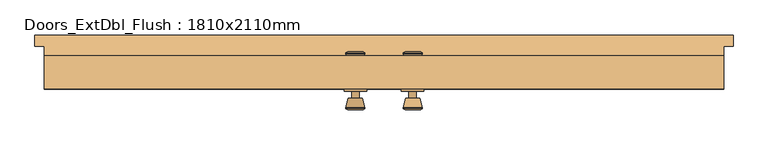
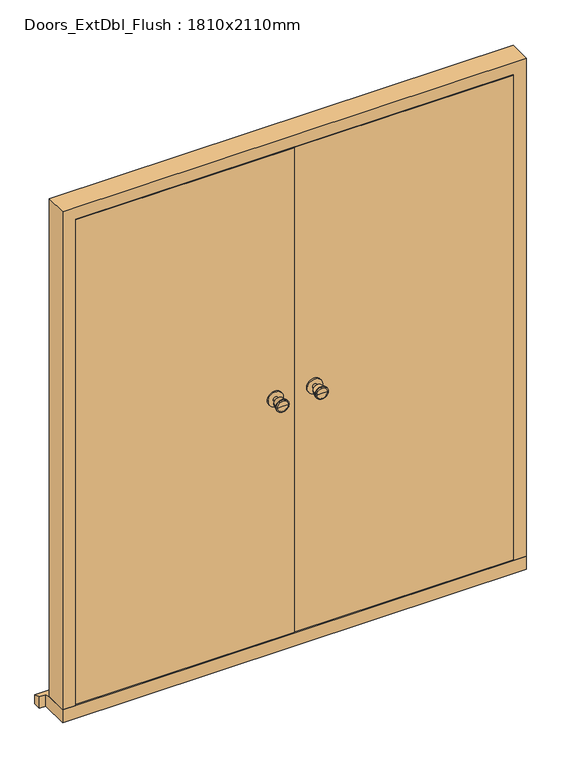
"""IFC4 building model written with IfcOpenShell, lengths in millimetres: door geometry, Doors_ExtDbl_Flush : 1810x2110mm."""

from ifc_helpers import new_model, si_unit, point, frame, frame_2d, origin, place, context, project, spatial, polyline, circle_curve, trimmed, segment, composite_curve, outline, extrude, faceted_brep, source, transform, mapped, element, save
from ifc_brep_helpers import plane_surface, cylinder_surface, revolved_surface, advanced_brep


def doors_extdbl_flush_1810x2110mm_a954e790(model_context):
    return source(origin(), model_context, "Body", "SolidModel", [
        advanced_brep(
        [(-76.5, -7.5, 1050.0), (-66.5, -7.5, 1050.0), (-86.5, -7.5, 1050.0), (-96.9758676, -56.5, 1050.0), (-56.0241324, -56.5, 1050.0), (-76.5, -56.5, 1050.0), (-101.5, -54.6721319, 1050.0), (-51.5, -54.6721319, 1050.0), (-101.5, -51.2084537, 1050.0), (-51.5, -51.2084537, 1050.0), (-95.136236, -26.5, 1050.0), (-57.863764, -26.5, 1050.0), (-86.5, -26.5, 1050.0), (-66.5, -26.5, 1050.0)],
        [
            (0, 1),
            (1, 2, circle_curve(frame((-76.5, -7.5, 1050.0), z_axis=(0.0, 1.0, 0.0), x_axis=(1.0, 0.0, 0.0)), 10.0)),
            (2, 0),
            (2, 1, circle_curve(frame((-76.5, -7.5, 1050.0), z_axis=(0.0, 1.0, 0.0), x_axis=(1.0, 0.0, 0.0)), 10.0)),
            (3, 4, circle_curve(frame((-76.5, -56.5, 1050.0), z_axis=(0.0, -1.0, 0.0), x_axis=(1.0, 0.0, 0.0)), 20.4758676)),
            (4, 5),
            (5, 3),
            (4, 3, circle_curve(frame((-76.5, -56.5, 1050.0), z_axis=(0.0, -1.0, 0.0), x_axis=(1.0, 0.0, 0.0)), 20.4758676)),
            (6, 7, circle_curve(frame((-76.5, -54.6721319, 1050.0), z_axis=(0.0, -1.0, 0.0), x_axis=(1.0, 0.0, 0.0)), 25.0)),
            (7, 4),
            (3, 6),
            (7, 6, circle_curve(frame((-76.5, -54.6721319, 1050.0), z_axis=(0.0, -1.0, 0.0), x_axis=(1.0, 0.0, 0.0)), 25.0)),
            (8, 9, circle_curve(frame((-76.5, -51.2084537, 1050.0), z_axis=(0.0, -1.0, 0.0), x_axis=(1.0, 0.0, 0.0)), 25.0)),
            (9, 7),
            (6, 8),
            (9, 8, circle_curve(frame((-76.5, -51.2084537, 1050.0), z_axis=(0.0, -1.0, 0.0), x_axis=(1.0, 0.0, 0.0)), 25.0)),
            (10, 11, circle_curve(frame((-76.5, -26.5, 1050.0), z_axis=(0.0, -1.0, 0.0), x_axis=(1.0, 0.0, 0.0)), 18.636236)),
            (11, 9),
            (8, 10),
            (11, 10, circle_curve(frame((-76.5, -26.5, 1050.0), z_axis=(0.0, -1.0, 0.0), x_axis=(1.0, 0.0, 0.0)), 18.636236)),
            (12, 13, circle_curve(frame((-76.5, -26.5, 1050.0), z_axis=(0.0, -1.0, 0.0), x_axis=(1.0, 0.0, 0.0)), 10.0)),
            (13, 11),
            (10, 12),
            (13, 12, circle_curve(frame((-76.5, -26.5, 1050.0), z_axis=(0.0, -1.0, 0.0), x_axis=(1.0, 0.0, 0.0)), 10.0)),
            (1, 13),
            (12, 2),
        ],
        [
            plane_surface(frame((-76.5, -7.5, 1050.0), z_axis=(0.0, 1.0, 0.0), x_axis=(1.0, 0.0, 0.0))),
            plane_surface(frame((-76.5, -56.5, 1050.0), z_axis=(0.0, -1.0, 0.0), x_axis=(1.0, 0.0, 0.0))),
            revolved_surface(polyline([(-56.0241324, -56.5, 1050.0), (-51.5, -54.6721319, 1050.0)]), (-76.5, -7.5, 1050.0), (0.0, 1.0, 0.0)),
            cylinder_surface(frame((-76.5, -7.5, 1050.0), z_axis=(0.0, 1.0, 0.0), x_axis=(1.0, 0.0, 0.0)), 25.0),
            revolved_surface(polyline([(-51.5, -51.2084537, 1050.0), (-57.863764, -26.5, 1050.0)]), (-76.5, -7.5, 1050.0), (0.0, 1.0, 0.0)),
            plane_surface(frame((-76.5, -26.5, 1050.0), z_axis=(0.0, 1.0, 0.0), x_axis=(1.0, 0.0, 0.0))),
            cylinder_surface(frame((-76.5, -7.5, 1050.0), z_axis=(0.0, 1.0, 0.0), x_axis=(1.0, 0.0, 0.0)), 10.0),
        ],
        [
            (0, [[1, 2, 3]]),
            (0, [[-3, 4, -1]]),
            (1, [[5, 6, 7]]),
            (1, [[8, -7, -6]]),
            (2, [[9, 10, -5, 11]]),
            (2, [[12, -11, -8, -10]]),
            (3, [[13, 14, -9, 15]]),
            (3, [[16, -15, -12, -14]]),
            (4, [[17, 18, -13, 19]]),
            (4, [[20, -19, -16, -18]]),
            (5, [[21, 22, -17, 23]]),
            (5, [[24, -23, -20, -22]]),
            (6, [[-2, 25, -21, 26]]),
            (6, [[-4, -26, -24, -25]]),
        ],
    ),
        extrude(outline(composite_curve([segment(trimmed(circle_curve(frame_2d((1050.0, -76.5)), 30.0), [point((1050.0, -46.5))], [point((1050.0, -106.5))], False, "CARTESIAN"), True, "CONTINUOUS"), segment(trimmed(circle_curve(frame_2d((1050.0, -76.5)), 30.0), [point((1050.0, -106.5))], [point((1050.0, -46.5))], False, "CARTESIAN"), True, "CONTINUOUS")], self_intersect=False)), frame((0.0, -7.5, 0.0), z_axis=(0.0, 1.0, 0.0), x_axis=(0.0, 0.0, 1.0)), (0.0, 0.0, 1.0), 6.0),
        advanced_brep(
        [(-76.5, 48.5, 1050.0), (-86.5, 48.5, 1050.0), (-66.5, 48.5, 1050.0), (-96.9758676, 97.5, 1050.0), (-76.5, 97.5, 1050.0), (-56.0241324, 97.5, 1050.0), (-101.5, 95.6721319, 1050.0), (-51.5, 95.6721319, 1050.0), (-101.5, 92.2084537, 1050.0), (-51.5, 92.2084537, 1050.0), (-95.136236, 67.5, 1050.0), (-57.863764, 67.5, 1050.0), (-86.5, 67.5, 1050.0), (-66.5, 67.5, 1050.0)],
        [
            (0, 1),
            (1, 2, circle_curve(frame((-76.5, 48.5, 1050.0), z_axis=(0.0, -1.0, 0.0), x_axis=(1.0, 0.0, 0.0)), 10.0)),
            (2, 0),
            (2, 1, circle_curve(frame((-76.5, 48.5, 1050.0), z_axis=(0.0, -1.0, 0.0), x_axis=(1.0, 0.0, 0.0)), 10.0)),
            (3, 4),
            (4, 5),
            (5, 3, circle_curve(frame((-76.5, 97.5, 1050.0), z_axis=(0.0, 1.0, 0.0), x_axis=(1.0, 0.0, 0.0)), 20.4758676)),
            (3, 5, circle_curve(frame((-76.5, 97.5, 1050.0), z_axis=(0.0, 1.0, 0.0), x_axis=(1.0, 0.0, 0.0)), 20.4758676)),
            (6, 3),
            (5, 7),
            (7, 6, circle_curve(frame((-76.5, 95.6721319, 1050.0), z_axis=(0.0, 1.0, 0.0), x_axis=(1.0, 0.0, 0.0)), 25.0)),
            (6, 7, circle_curve(frame((-76.5, 95.6721319, 1050.0), z_axis=(0.0, 1.0, 0.0), x_axis=(1.0, 0.0, 0.0)), 25.0)),
            (8, 6),
            (7, 9),
            (9, 8, circle_curve(frame((-76.5, 92.2084537, 1050.0), z_axis=(0.0, 1.0, 0.0), x_axis=(1.0, 0.0, 0.0)), 25.0)),
            (8, 9, circle_curve(frame((-76.5, 92.2084537, 1050.0), z_axis=(0.0, 1.0, 0.0), x_axis=(1.0, 0.0, 0.0)), 25.0)),
            (10, 8),
            (9, 11),
            (11, 10, circle_curve(frame((-76.5, 67.5, 1050.0), z_axis=(0.0, 1.0, 0.0), x_axis=(1.0, 0.0, 0.0)), 18.636236)),
            (10, 11, circle_curve(frame((-76.5, 67.5, 1050.0), z_axis=(0.0, 1.0, 0.0), x_axis=(1.0, 0.0, 0.0)), 18.636236)),
            (12, 10),
            (11, 13),
            (13, 12, circle_curve(frame((-76.5, 67.5, 1050.0), z_axis=(0.0, 1.0, 0.0), x_axis=(1.0, 0.0, 0.0)), 10.0)),
            (12, 13, circle_curve(frame((-76.5, 67.5, 1050.0), z_axis=(0.0, 1.0, 0.0), x_axis=(1.0, 0.0, 0.0)), 10.0)),
            (1, 12),
            (13, 2),
        ],
        [
            plane_surface(frame((-76.5, 48.5, 1050.0), z_axis=(0.0, -1.0, 0.0), x_axis=(1.0, 0.0, 0.0))),
            plane_surface(frame((-76.5, 97.5, 1050.0), z_axis=(0.0, 1.0, 0.0), x_axis=(1.0, 0.0, 0.0))),
            revolved_surface(polyline([(-56.0241324, 97.5, 1050.0), (-51.5, 95.6721319, 1050.0)]), (-76.5, 48.5, 1050.0), (0.0, -1.0, 0.0)),
            cylinder_surface(frame((-76.5, 48.5, 1050.0), z_axis=(0.0, -1.0, 0.0), x_axis=(1.0, 0.0, 0.0)), 25.0),
            revolved_surface(polyline([(-51.5, 92.2084537, 1050.0), (-57.863764, 67.5, 1050.0)]), (-76.5, 48.5, 1050.0), (0.0, -1.0, 0.0)),
            plane_surface(frame((-76.5, 67.5, 1050.0), z_axis=(0.0, -1.0, 0.0), x_axis=(1.0, 0.0, 0.0))),
            cylinder_surface(frame((-76.5, 48.5, 1050.0), z_axis=(0.0, -1.0, 0.0), x_axis=(1.0, 0.0, 0.0)), 10.0),
        ],
        [
            (0, [[1, 2, 3]]),
            (0, [[-3, 4, -1]]),
            (1, [[5, 6, 7]]),
            (1, [[-6, -5, 8]]),
            (2, [[9, -7, 10, 11]]),
            (2, [[-10, -8, -9, 12]]),
            (3, [[13, -11, 14, 15]]),
            (3, [[-14, -12, -13, 16]]),
            (4, [[17, -15, 18, 19]]),
            (4, [[-18, -16, -17, 20]]),
            (5, [[21, -19, 22, 23]]),
            (5, [[-22, -20, -21, 24]]),
            (6, [[25, -23, 26, -2]]),
            (6, [[-26, -24, -25, -4]]),
        ],
    ),
        extrude(outline(composite_curve([segment(trimmed(circle_curve(frame_2d((1050.0, -76.5)), 30.0), [point((1050.0, -46.5))], [point((1050.0, -106.5))], False, "CARTESIAN"), True, "CONTINUOUS"), segment(trimmed(circle_curve(frame_2d((1050.0, -76.5)), 30.0), [point((1050.0, -106.5))], [point((1050.0, -46.5))], False, "CARTESIAN"), True, "CONTINUOUS")], self_intersect=False)), frame((0.0, 42.5, 0.0), z_axis=(0.0, 1.0, 0.0), x_axis=(0.0, 0.0, 1.0)), (0.0, 0.0, 1.0), 6.0),
        advanced_brep(
        [(76.5, -7.5, 1050.0), (86.5, -7.5, 1050.0), (66.5, -7.5, 1050.0), (96.9758676, -56.5, 1050.0), (76.5, -56.5, 1050.0), (56.0241324, -56.5, 1050.0), (101.5, -54.6721319, 1050.0), (51.5, -54.6721319, 1050.0), (101.5, -51.2084537, 1050.0), (51.5, -51.2084537, 1050.0), (95.136236, -26.5, 1050.0), (57.863764, -26.5, 1050.0), (86.5, -26.5, 1050.0), (66.5, -26.5, 1050.0)],
        [
            (0, 1),
            (1, 2, circle_curve(frame((76.5, -7.5, 1050.0), z_axis=(0.0, 1.0, 0.0), x_axis=(-1.0, 0.0, 0.0)), 10.0)),
            (2, 0),
            (2, 1, circle_curve(frame((76.5, -7.5, 1050.0), z_axis=(0.0, 1.0, 0.0), x_axis=(-1.0, 0.0, 0.0)), 10.0)),
            (3, 4),
            (4, 5),
            (5, 3, circle_curve(frame((76.5, -56.5, 1050.0), z_axis=(0.0, -1.0, 0.0), x_axis=(-1.0, 0.0, 0.0)), 20.4758676)),
            (3, 5, circle_curve(frame((76.5, -56.5, 1050.0), z_axis=(0.0, -1.0, 0.0), x_axis=(-1.0, 0.0, 0.0)), 20.4758676)),
            (6, 3),
            (5, 7),
            (7, 6, circle_curve(frame((76.5, -54.6721319, 1050.0), z_axis=(0.0, -1.0, 0.0), x_axis=(-1.0, 0.0, 0.0)), 25.0)),
            (6, 7, circle_curve(frame((76.5, -54.6721319, 1050.0), z_axis=(0.0, -1.0, 0.0), x_axis=(-1.0, 0.0, 0.0)), 25.0)),
            (8, 6),
            (7, 9),
            (9, 8, circle_curve(frame((76.5, -51.2084537, 1050.0), z_axis=(0.0, -1.0, 0.0), x_axis=(-1.0, 0.0, 0.0)), 25.0)),
            (8, 9, circle_curve(frame((76.5, -51.2084537, 1050.0), z_axis=(0.0, -1.0, 0.0), x_axis=(-1.0, 0.0, 0.0)), 25.0)),
            (10, 8),
            (9, 11),
            (11, 10, circle_curve(frame((76.5, -26.5, 1050.0), z_axis=(0.0, -1.0, 0.0), x_axis=(-1.0, 0.0, 0.0)), 18.636236)),
            (10, 11, circle_curve(frame((76.5, -26.5, 1050.0), z_axis=(0.0, -1.0, 0.0), x_axis=(-1.0, 0.0, 0.0)), 18.636236)),
            (12, 10),
            (11, 13),
            (13, 12, circle_curve(frame((76.5, -26.5, 1050.0), z_axis=(0.0, -1.0, 0.0), x_axis=(-1.0, 0.0, 0.0)), 10.0)),
            (12, 13, circle_curve(frame((76.5, -26.5, 1050.0), z_axis=(0.0, -1.0, 0.0), x_axis=(-1.0, 0.0, 0.0)), 10.0)),
            (1, 12),
            (13, 2),
        ],
        [
            plane_surface(frame((76.5, -7.5, 1050.0), z_axis=(0.0, 1.0, 0.0), x_axis=(-1.0, 0.0, 0.0))),
            plane_surface(frame((76.5, -56.5, 1050.0), z_axis=(0.0, -1.0, 0.0), x_axis=(-1.0, 0.0, 0.0))),
            revolved_surface(polyline([(56.0241324, -56.5, 1050.0), (51.5, -54.6721319, 1050.0)]), (76.5, -7.5, 1050.0), (0.0, 1.0, 0.0)),
            cylinder_surface(frame((76.5, -7.5, 1050.0), z_axis=(0.0, 1.0, 0.0), x_axis=(-1.0, 0.0, 0.0)), 25.0),
            revolved_surface(polyline([(51.5, -51.2084537, 1050.0), (57.863764, -26.5, 1050.0)]), (76.5, -7.5, 1050.0), (0.0, 1.0, 0.0)),
            plane_surface(frame((76.5, -26.5, 1050.0), z_axis=(0.0, 1.0, 0.0), x_axis=(-1.0, 0.0, 0.0))),
            cylinder_surface(frame((76.5, -7.5, 1050.0), z_axis=(0.0, 1.0, 0.0), x_axis=(-1.0, 0.0, 0.0)), 10.0),
        ],
        [
            (0, [[1, 2, 3]]),
            (0, [[-3, 4, -1]]),
            (1, [[5, 6, 7]]),
            (1, [[-6, -5, 8]]),
            (2, [[9, -7, 10, 11]]),
            (2, [[-10, -8, -9, 12]]),
            (3, [[13, -11, 14, 15]]),
            (3, [[-14, -12, -13, 16]]),
            (4, [[17, -15, 18, 19]]),
            (4, [[-18, -16, -17, 20]]),
            (5, [[21, -19, 22, 23]]),
            (5, [[-22, -20, -21, 24]]),
            (6, [[25, -23, 26, -2]]),
            (6, [[-26, -24, -25, -4]]),
        ],
    ),
        extrude(outline(composite_curve([segment(trimmed(circle_curve(frame_2d((1050.0, 76.5)), 30.0), [point((1050.0, 46.5))], [point((1050.0, 106.5))], False, "CARTESIAN"), True, "CONTINUOUS"), segment(trimmed(circle_curve(frame_2d((1050.0, 76.5)), 30.0), [point((1050.0, 106.5))], [point((1050.0, 46.5))], False, "CARTESIAN"), True, "CONTINUOUS")], self_intersect=False)), frame((0.0, -7.5, 0.0), z_axis=(0.0, 1.0, 0.0), x_axis=(0.0, 0.0, 1.0)), (0.0, 0.0, 1.0), 6.0),
        advanced_brep(
        [(76.5, 48.5, 1050.0), (66.5, 48.5, 1050.0), (86.5, 48.5, 1050.0), (96.9758676, 97.5, 1050.0), (56.0241324, 97.5, 1050.0), (76.5, 97.5, 1050.0), (101.5, 95.6721319, 1050.0), (51.5, 95.6721319, 1050.0), (101.5, 92.2084537, 1050.0), (51.5, 92.2084537, 1050.0), (95.136236, 67.5, 1050.0), (57.863764, 67.5, 1050.0), (86.5, 67.5, 1050.0), (66.5, 67.5, 1050.0)],
        [
            (0, 1),
            (1, 2, circle_curve(frame((76.5, 48.5, 1050.0), z_axis=(0.0, -1.0, 0.0), x_axis=(-1.0, 0.0, 0.0)), 10.0)),
            (2, 0),
            (2, 1, circle_curve(frame((76.5, 48.5, 1050.0), z_axis=(0.0, -1.0, 0.0), x_axis=(-1.0, 0.0, 0.0)), 10.0)),
            (3, 4, circle_curve(frame((76.5, 97.5, 1050.0), z_axis=(0.0, 1.0, 0.0), x_axis=(-1.0, 0.0, 0.0)), 20.4758676)),
            (4, 5),
            (5, 3),
            (4, 3, circle_curve(frame((76.5, 97.5, 1050.0), z_axis=(0.0, 1.0, 0.0), x_axis=(-1.0, 0.0, 0.0)), 20.4758676)),
            (6, 7, circle_curve(frame((76.5, 95.6721319, 1050.0), z_axis=(0.0, 1.0, 0.0), x_axis=(-1.0, 0.0, 0.0)), 25.0)),
            (7, 4),
            (3, 6),
            (7, 6, circle_curve(frame((76.5, 95.6721319, 1050.0), z_axis=(0.0, 1.0, 0.0), x_axis=(-1.0, 0.0, 0.0)), 25.0)),
            (8, 9, circle_curve(frame((76.5, 92.2084537, 1050.0), z_axis=(0.0, 1.0, 0.0), x_axis=(-1.0, 0.0, 0.0)), 25.0)),
            (9, 7),
            (6, 8),
            (9, 8, circle_curve(frame((76.5, 92.2084537, 1050.0), z_axis=(0.0, 1.0, 0.0), x_axis=(-1.0, 0.0, 0.0)), 25.0)),
            (10, 11, circle_curve(frame((76.5, 67.5, 1050.0), z_axis=(0.0, 1.0, 0.0), x_axis=(-1.0, 0.0, 0.0)), 18.636236)),
            (11, 9),
            (8, 10),
            (11, 10, circle_curve(frame((76.5, 67.5, 1050.0), z_axis=(0.0, 1.0, 0.0), x_axis=(-1.0, 0.0, 0.0)), 18.636236)),
            (12, 13, circle_curve(frame((76.5, 67.5, 1050.0), z_axis=(0.0, 1.0, 0.0), x_axis=(-1.0, 0.0, 0.0)), 10.0)),
            (13, 11),
            (10, 12),
            (13, 12, circle_curve(frame((76.5, 67.5, 1050.0), z_axis=(0.0, 1.0, 0.0), x_axis=(-1.0, 0.0, 0.0)), 10.0)),
            (1, 13),
            (12, 2),
        ],
        [
            plane_surface(frame((76.5, 48.5, 1050.0), z_axis=(0.0, -1.0, 0.0), x_axis=(-1.0, 0.0, 0.0))),
            plane_surface(frame((76.5, 97.5, 1050.0), z_axis=(0.0, 1.0, 0.0), x_axis=(-1.0, 0.0, 0.0))),
            revolved_surface(polyline([(56.0241324, 97.5, 1050.0), (51.5, 95.6721319, 1050.0)]), (76.5, 48.5, 1050.0), (0.0, -1.0, 0.0)),
            cylinder_surface(frame((76.5, 48.5, 1050.0), z_axis=(0.0, -1.0, 0.0), x_axis=(-1.0, 0.0, 0.0)), 25.0),
            revolved_surface(polyline([(51.5, 92.2084537, 1050.0), (57.863764, 67.5, 1050.0)]), (76.5, 48.5, 1050.0), (0.0, -1.0, 0.0)),
            plane_surface(frame((76.5, 67.5, 1050.0), z_axis=(0.0, -1.0, 0.0), x_axis=(-1.0, 0.0, 0.0))),
            cylinder_surface(frame((76.5, 48.5, 1050.0), z_axis=(0.0, -1.0, 0.0), x_axis=(-1.0, 0.0, 0.0)), 10.0),
        ],
        [
            (0, [[1, 2, 3]]),
            (0, [[-3, 4, -1]]),
            (1, [[5, 6, 7]]),
            (1, [[8, -7, -6]]),
            (2, [[9, 10, -5, 11]]),
            (2, [[12, -11, -8, -10]]),
            (3, [[13, 14, -9, 15]]),
            (3, [[16, -15, -12, -14]]),
            (4, [[17, 18, -13, 19]]),
            (4, [[20, -19, -16, -18]]),
            (5, [[21, 22, -17, 23]]),
            (5, [[24, -23, -20, -22]]),
            (6, [[-2, 25, -21, 26]]),
            (6, [[-4, -26, -24, -25]]),
        ],
    ),
        extrude(outline(composite_curve([segment(trimmed(circle_curve(frame_2d((1050.0, 76.5)), 30.0), [point((1050.0, 46.5))], [point((1050.0, 106.5))], False, "CARTESIAN"), True, "CONTINUOUS"), segment(trimmed(circle_curve(frame_2d((1050.0, 76.5)), 30.0), [point((1050.0, 106.5))], [point((1050.0, 46.5))], False, "CARTESIAN"), True, "CONTINUOUS")], self_intersect=False)), frame((0.0, 42.5, 0.0), z_axis=(0.0, 1.0, 0.0), x_axis=(0.0, 0.0, 1.0)), (0.0, 0.0, 1.0), 6.0),
        faceted_brep([(834.5, 87.5, 54.5), (905.0, 87.5, 54.5), (905.0, -1.5, 54.5), (856.5, -1.5, 54.5), (856.5, 45.5, 54.5), (834.5, 45.5, 54.5), (834.5, 87.5, 2039.5), (-834.5, 87.5, 2039.5), (-834.5, 87.5, 54.5), (-905.0, 87.5, 54.5), (-905.0, 87.5, 2110.0), (905.0, 87.5, 2110.0), (905.0, -1.5, 2110.0), (-905.0, -1.5, 2110.0), (-905.0, -1.5, 54.5), (-856.5, -1.5, 54.5), (-856.5, -1.5, 2061.5), (856.5, -1.5, 2061.5), (856.5, 45.5, 2061.5), (-856.5, 45.5, 2061.5), (-856.5, 45.5, 54.5), (-834.5, 45.5, 54.5), (-834.5, 45.5, 2039.5), (834.5, 45.5, 2039.5)], [[[0, 1, 2, 3, 4, 5]], [[1, 0, 6, 7, 8, 9, 10, 11]], [[2, 1, 11, 12]], [[3, 2, 12, 13, 14, 15, 16, 17]], [[4, 3, 17, 18]], [[5, 4, 18, 19, 20, 21, 22, 23]], [[0, 5, 23, 6]], [[12, 11, 10, 13]], [[18, 17, 16, 19]], [[6, 23, 22, 7]], [[8, 21, 20, 15, 14, 9]], [[13, 10, 9, 14]], [[19, 16, 15, 20]], [[7, 22, 21, 8]]]),
        faceted_brep([(930.0, 142.5, 0.0), (930.0, 142.5, 38.5947221), (930.0, 112.5, 47.2703282), (930.0, 112.5, 0.0), (-930.0, 142.5, 38.5947221), (-930.0, 142.5, 0.0), (-930.0, 112.5, 0.0), (-930.0, 112.5, 47.2703282), (905.0, 112.5, 0.0), (905.0, -1.5, 0.0), (-905.0, -1.5, 0.0), (-905.0, 112.5, 0.0), (-905.0, 112.5, 47.2703282), (-905.0, 87.5, 54.5), (905.0, 87.5, 54.5), (905.0, 112.5, 47.2703282), (-905.0, -1.5, 54.5), (905.0, -1.5, 54.5)], [[[0, 1, 2, 3]], [[4, 5, 6, 7]], [[5, 0, 3, 8, 9, 10, 11, 6]], [[1, 0, 5, 4]], [[1, 4, 7, 12, 13, 14, 15, 2]], [[13, 16, 17, 14]], [[16, 10, 9, 17]], [[12, 11, 10, 16, 13]], [[11, 12, 7, 6]], [[8, 15, 14, 17, 9]], [[15, 8, 3, 2]]]),
        extrude(outline(polyline([(853.5, -1.5), (1.5, -1.5), (1.5, 42.5), (853.5, 42.5), (853.5, -1.5)])), frame((0.0, 0.0, 58.5), z_axis=(0.0, 0.0, 1.0), x_axis=(1.0, 0.0, 0.0)), (0.0, 0.0, 1.0), 2000.0),
        extrude(outline(polyline([(-1.5, -1.5), (-853.5, -1.5), (-853.5, 42.5), (-1.5, 42.5), (-1.5, -1.5)])), frame((0.0, 0.0, 58.5), z_axis=(0.0, 0.0, 1.0), x_axis=(1.0, 0.0, 0.0)), (0.0, 0.0, 1.0), 2000.0),
    ])


if __name__ == "__main__":
    model = new_model("IFC4")
    model_context = context("Model", 3, world=origin())
    ifc_project = project(units=[si_unit("LENGTHUNIT", "METRE", prefix="MILLI")], contexts=[model_context])
    site = spatial("IfcSite", under=ifc_project)
    building = spatial("IfcBuilding", under=site)
    placement = place(None, origin())
    doors_extdbl_flush_1810x2110mm_shape = doors_extdbl_flush_1810x2110mm_a954e790(model_context)
    element("IfcDoor", 1, ObjectType="Doors_ExtDbl_Flush : 1810x2110mm", at=placement, inside=building, context=model_context, shape_type="MappedRepresentation", body=[
        mapped(doors_extdbl_flush_1810x2110mm_shape, transform((0.0, 0.0, 0.0), x_axis=(1.0, 0.0, 0.0), y_axis=(0.0, 1.0, 0.0), z_axis=(0.0, 0.0, 1.0))),
    ])
    save(model, "model.ifc")

# Revit data of these elements
# Type "Doors_ExtDbl_Flush : 1810x2110mm"
#   Type Mark = "44"
#   Type Comments = "External Double"
#   Operation = "DoubleDoorSingleSwing"
#   Keynote = "L20"
#   Analytic Construction = "Metal"
#   Wrap Layers (Ext) from Ext = 102.5 mm
#   Wrap Layers (Int) from Ext = 177.5 mm
#   Thickness = 44 mm
#   Rough Width = 1810 mm
#   Rough Height = 2110 mm
#   O/A Frame Width = 64 mm
#   Heat Transfer Coefficient (U) = 3.7021 W/(m²·K)
#   Handle Z Distance = 1050 mm
#   FrameWidth = 42 mm
#   FrameOffset - External = 25 mm
#   FrameDepth = 89 mm
#   Door Panel Width = 852 mm
#   Door Panel Thickness = 44 mm
#   Door Panel Height = 2000 mm
#   Cill Thickness = 54.5 mm
#   Cill Projection = 30 mm
#   Handle X Distance = 75 mm
#   Height = 2110 mm
#   Structural Tolerance = 6.5 mm
#   Tolerance = 3 mm
#   Undercut = 4 mm
#   Width = 1810 mm
#   Cill Extension = 25 mm
#   Cavity Closer Width = 50 mm
#   Cavity Closer Offset from Ext = 102.5 mm
#   Cavity Closer Depth = 85 mm
#   Define Thermal Properties by = 0
#   Vis - Ironmongery = yes
#   Vis - Cavity Closers = yes
#   Function = 1
#   Material Door = Door - Panel
#   Material Frame = Door - Frame/Mullion
#   Material Ironmongery = Door - Handle
#   Visual Light Transmittance = 0
#   Thermal Resistance (R) = 0
#   Solar Heat Gain Coefficient = 0
#   Wall Closure = (empty or 0)
# Element 1 (IfcDoor, "Doors_ExtDbl_Flush : 1810x2110mm")
#   Materials on its faces: "Door - Handle", "Door - Frame/Mullion", "Door - Panel"
# Materials
#   "Door - Panel": class "Wood", colour RGB 210 159 95, transparency 0, Keynote = "L20", Cost = 0
#   "Door - Frame/Mullion": class "Wood", colour RGB 212 179 113, transparency 0, Keynote = "L20", Cost = 0
#   "Door - Handle": colour RGB 0 0 0, transparency 0, Keynote = "P21", Cost = 0
